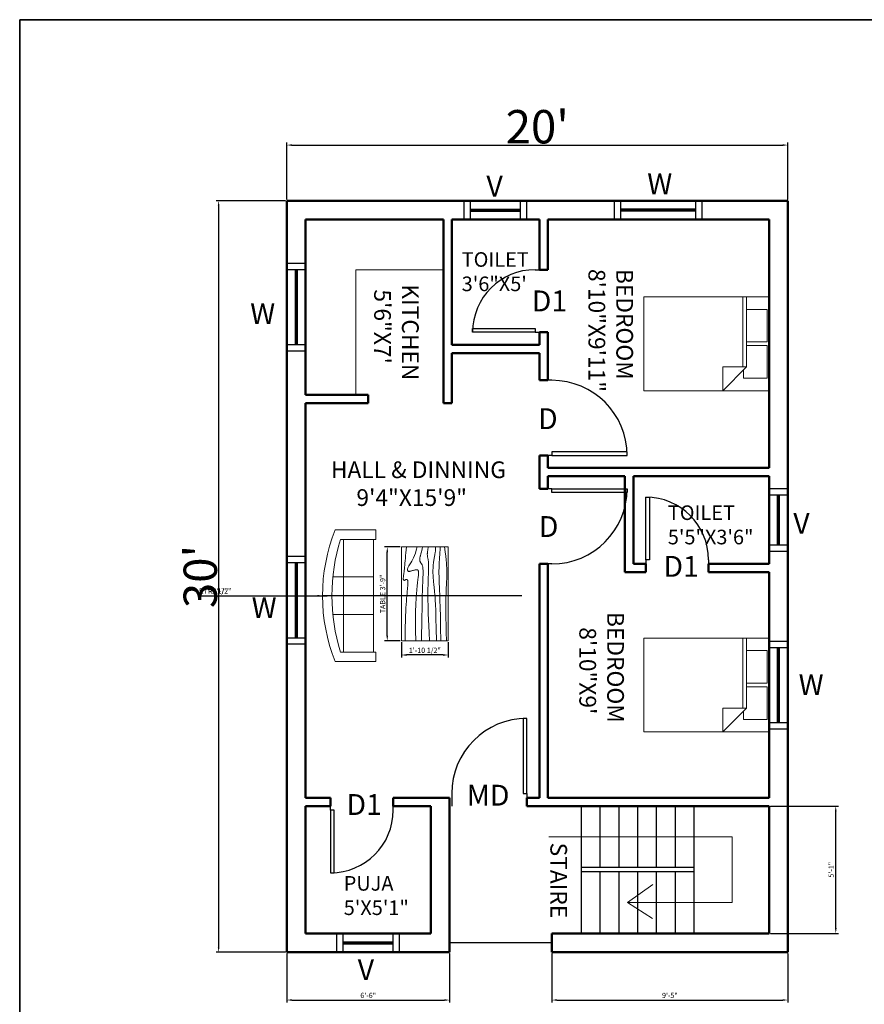
# Model space of a CAD drawing. Units: inches. Extents: x 2150 to 10686, y 1035 to 5077.
# Tile 8 of 12: x 6113 to 6517, y 4605 to 5077. Entities that reach past the tile are written whole.
import ezdxf

# ---------------------------------------------------------------- set-up
doc = ezdxf.new("R2010")
doc.units = ezdxf.units.IN
for name, color, linetype, lineweight in [('A-ANNO-DIMS', 2, 'Continuous', 18), ('A-ANNO-IDEN', 2, 'Continuous', 18), ('A-ANNO-SYMB', 3, 'Continuous', 18), ('A-ANNO-TTLB', 7, 'Continuous', 35), ('A-AREA-IDEN', 7, 'Continuous', 18), ('A-DOOR', 4, 'Continuous', 25), ('A-FLOR-FIXT', 9, 'Continuous', 18), ('A-FLOR-STRS', 4, 'Continuous', 25), ('A-FURN', 8, 'Continuous', 18), ('A-GLAZ', 30, 'Continuous', 25), ('A-WALL', 18, 'Continuous', 50)]:
    doc.layers.add(name, color=color, linetype=linetype, lineweight=lineweight)
doc.styles.get("Standard").update_dxf_attribs({"font": 'arial.ttf'})
doc.dimstyles.new('ISO-25', dxfattribs={"dimtxt": 2.5, "dimasz": 2.5, "dimexe": 1.25, "dimexo": 0.625, "dimtad": 1, "dimdec": 0, "dimlunit": 3, "dimtxsty": 'Standard', "dimcen": 2.5, "dimadec": 0, "dimazin": 0, "dimtfac": 1, "dimtdec": 0, "dimtmove": 0, "dimatfit": 3, "dimfxl": 1, "dimarcsym": 0})

# ---------------------------------------------------------------- blocks, each defined once
blk = doc.blocks.new('*U9')
for p, q in [((0, 0), (0, -6)), ((-36, 0), (-36, -6))]:
    blk.add_line(p, q)
blk.add_lwpolyline([(0, 0), (0, 36), (-1.75, 36), (-1.75, 0)], close=True)
blk.add_arc((0, 0), 36, 90, 180)
blk = doc.blocks.new('*U18')
for p, q in [((0, 0), (0, -6)), ((30, 0), (30, -6))]:
    blk.add_line(p, q)
blk.add_lwpolyline([(0, 0), (0, 30), (1.75, 30), (1.75, 0)], close=True)
blk.add_arc((0, 0), 30, 0, 90)
blk = doc.blocks.new('*U19')
for p, q in [((0, 0), (0, -6)), ((36, 0), (36, -6))]:
    blk.add_line(p, q)
blk.add_lwpolyline([(0, 0), (0, 36), (1.75, 36), (1.75, 0)], close=True)
blk.add_arc((0, 0), 36, 0, 90)
blk = doc.blocks.new('*U20')
for p, q in [((-30, 0), (-30, 6)), ((0, 0), (0, 6))]:
    blk.add_line(p, q)
blk.add_lwpolyline([(0, 0), (0, -30), (-1.75, -30), (-1.75, 0)], close=True)
blk.add_arc((0, 0), 30, 180, 270)
blk = doc.blocks.new('*U21')
for p, q in [((0, 0), (0, 6)), ((30, 0), (30, 6))]:
    blk.add_line(p, q)
blk.add_lwpolyline([(0, 0), (0, -30), (1.75, -30), (1.75, 0)], close=True)
blk.add_arc((0, 0), 30, 270, 0)
blk = doc.blocks.new('Bed - Queen')
for p, q in [((0, -80.00003), (0, 0)), ((0, 0), (59.99999, 0)), ((59.99999, 0), (59.99999, -80.00003)), ((7.99999, -1.2), (28.79998, -1.2)), ((7.99999, -14.4), (7.99999, -1.2)), ((28.79998, -1.2), (28.79998, -14.4)), ((31.19999, -1.2), (51.99999, -1.2)), ((31.19999, -14.4), (31.19999, -1.2)), ((51.99999, -1.2), (51.99999, -16.4)), ((0, -14.4), (44.8, -14.4)), ((44.8, -16.8), (0, -16.8)), ((59.99999, -29.6), (44.8, -14.4)), ((44.8, -14.4), (44.8, -29.6)), ((51.99999, -16.4), (46.79936, -16.4)), ((44.8, -29.6), (59.99999, -29.6)), ((59.99999, -80.00003), (0, -80.00003))]:
    blk.add_line(p, q)
blk = doc.blocks.new('Sofa - Roundback 7 ft.')
for p, q in [((-36.000027, -34), (-36.000027, -11.4696)), ((-12.00002, -32.4421), (-12.00003, -6.5971)), ((11.99997, -32.4421), (11.99998, -6.5971)), ((35.99998, -34), (35.99998, -11.4696)), ((-35.999844, -13.3819), (35.9998, -13.3819)), ((-36.000027, -32.4421), (35.99998, -32.4421))]:
    blk.add_line(p, q)
for points in [[(-36.000027, -34), (-42.000027, -34), (-42.000027, -8)], [(41.99998, -8), (41.99998, -34), (35.99998, -34)]]:
    blk.add_lwpolyline(points)
for centre, radius, start, end in [((0, -114.25), 114.25, 68.43141, 111.5686), ((-0.00001, -127.1968), 121.1968, 72.72033, 107.2797)]:
    blk.add_arc(centre, radius, start, end)
blk = doc.blocks.new('Table - Rectangular Woodgrain 60 x 30 in.')
for p, q in [((0, 0), (0, -30)), ((60, 0), (0, 0)), ((60, -30), (60, 0)), ((0, -30), (60, -30))]:
    blk.add_line(p, q)
for points in [[(0, -2.4), (4.8155, -2.418), (9.0302, -2.4688), (12.709, -2.5477), (15.9167, -2.65), (18.7181, -2.7711), (21.1781, -2.9063), (23.3616, -3.0508), (25.3333, -3.2), (27.1477, -3.3495), (28.8172, -3.4958), (30.3437, -3.636), (31.7291, -3.7667), (32.9756, -3.8849), (34.0849, -3.9875), (35.059, -4.0714), (35.9, -4.1334), (36.6114, -4.1711), (37.2041, -4.1854), (37.6906, -4.1779), (38.0833, -4.15), (38.3948, -4.1034), (38.6375, -4.0396), (38.8239, -3.9602), (38.9666, -3.8667), (39.0764, -3.7608), (39.1573, -3.6448), (39.2116, -3.521), (39.2416, -3.3917), (39.2498, -3.2593), (39.2385, -3.1261), (39.21, -2.9944), (39.1666, -2.8667), (39.111, -2.7447), (39.0468, -2.6281), (38.978, -2.5163), (38.9083, -2.4083), (38.8418, -2.3035), (38.7823, -2.201), (38.7337, -2.1001), (38.7, -2), (38.6844, -1.9003), (38.6875, -1.8021), (38.7094, -1.707), (38.75, -1.6167), (38.8094, -1.5326), (38.8875, -1.4563), (38.9844, -1.3893), (39.1, -1.3333), (39.2351, -1.2896), (39.3937, -1.2583), (39.5804, -1.2396), (39.8, -1.2333), (40.057, -1.2396), (40.3562, -1.2583), (40.7023, -1.2896), (41.1, -1.3333), (41.5547, -1.3895), (42.0755, -1.4573), (42.6721, -1.5361), (43.3542, -1.625), (44.1316, -1.7233), (45.014, -1.8302), (46.0114, -1.9449), (47.1333, -2.0667), (48.3862, -2.1947), (49.7625, -2.3281), (51.2513, -2.4663), (52.8416, -2.6083), (54.5226, -2.7535), (56.2833, -2.9011), (58.1127, -3.0501), (60, -3.2)], [(0, -9.2), (6.5759, -9.0858), (11.9385, -9.0365), (16.2527, -9.0418), (19.6833, -9.0917), (22.3952, -9.1759), (24.5531, -9.2844), (26.322, -9.4069), (27.8666, -9.5333), (29.3241, -9.6553), (30.7203, -9.7719), (32.0532, -9.8837), (33.3208, -9.9917), (34.5213, -10.0965), (35.6526, -10.199), (36.7128, -10.2999), (37.7, -10.4), (38.6129, -10.4996), (39.4531, -10.5969), (40.223, -10.6895), (40.925, -10.775), (41.5613, -10.8512), (42.1344, -10.9156), (42.6465, -10.966), (43.1, -11), (43.4976, -11.0158), (43.8437, -11.0136), (44.143, -10.9942), (44.4, -10.9583), (44.6195, -10.9069), (44.8062, -10.8406), (44.9648, -10.7603), (45.1, -10.6667), (45.2155, -10.5598), (45.3114, -10.4365), (45.3871, -10.2929), (45.4416, -10.125), (45.4743, -9.929), (45.4844, -9.7011), (45.4709, -9.4371), (45.4333, -9.1333), (45.3716, -8.7883), (45.2896, -8.4104), (45.1919, -8.0107), (45.0833, -7.6), (44.9685, -7.1893), (44.8521, -6.7896), (44.7388, -6.4117), (44.6333, -6.0667), (44.54, -5.7628), (44.4614, -5.4979), (44.4001, -5.2675), (44.3583, -5.0667), (44.3384, -4.8909), (44.3427, -4.7354), (44.3736, -4.5956), (44.4333, -4.4667), (44.5236, -4.3453), (44.6427, -4.2333), (44.7884, -4.1339), (44.9583, -4.05), (45.1501, -3.9849), (45.3614, -3.9417), (45.59, -3.9234), (45.8333, -3.9333), (46.0915, -3.9749), (46.3734, -4.0531), (46.6906, -4.1736), (47.0542, -4.3417), (47.4756, -4.5629), (47.9661, -4.8427), (48.5372, -5.1866), (49.2, -5.6), (49.9676, -6.0844), (50.8594, -6.625), (51.8965, -7.2031), (53.1, -7.8), (54.491, -8.3969), (56.0906, -8.975), (57.9199, -9.5156), (60, -10)], [(0, -12.8), (5.1847, -12.9322), (9.6213, -13.0323), (13.3963, -13.1059), (16.5958, -13.1583), (19.3063, -13.1952), (21.614, -13.2219), (23.6054, -13.2439), (25.3666, -13.2667), (26.9728, -13.2947), (28.4531, -13.3281), (29.8256, -13.3663), (31.1083, -13.4083), (32.3191, -13.4535), (33.476, -13.501), (34.597, -13.5501), (35.7, -13.6), (36.7984, -13.6497), (37.8875, -13.6979), (38.9578, -13.743), (40, -13.7833), (41.0047, -13.8174), (41.9625, -13.8438), (42.864, -13.8607), (43.7, -13.8667), (44.4631, -13.8604), (45.1552, -13.8417), (45.7801, -13.8104), (46.3416, -13.7667), (46.8439, -13.7104), (47.2906, -13.6417), (47.6858, -13.5604), (48.0333, -13.4667), (48.3375, -13.3608), (48.6042, -13.2448), (48.8396, -13.121), (49.05, -12.9917), (49.2417, -12.8593), (49.4208, -12.7261), (49.5937, -12.5944), (49.7667, -12.4667), (49.9452, -12.3451), (50.1323, -12.2313), (50.3303, -12.1268), (50.5416, -12.0333), (50.7686, -11.9524), (51.0135, -11.8854), (51.2788, -11.8341), (51.5666, -11.8), (51.8785, -11.7843), (52.2116, -11.7865), (52.562, -11.8059), (52.926, -11.8417), (53.2998, -11.8931), (53.6795, -11.9594), (54.0614, -12.0397), (54.4416, -12.1333), (54.8223, -12.2401), (55.2293, -12.3625), (55.6942, -12.5037), (56.2489, -12.6667), (56.9251, -12.8547), (57.7545, -13.0708), (58.7689, -13.3182), (60, -13.6)], [(0, -18), (5.124, -17.7273), (9.6609, -17.5057), (13.6705, -17.3303), (17.2125, -17.1958), (20.3467, -17.0973), (23.1328, -17.0297), (25.6307, -16.9878), (27.9, -16.9667), (29.9928, -16.9617), (31.9302, -16.9703), (33.7254, -16.9907), (35.3917, -17.0208), (36.9423, -17.0588), (38.3906, -17.1026), (39.7499, -17.1503), (41.0333, -17.2), (42.2519, -17.2496), (43.4073, -17.2969), (44.4986, -17.3395), (45.525, -17.375), (46.4858, -17.4012), (47.3802, -17.4156), (48.2074, -17.416), (48.9667, -17.4), (49.6583, -17.3662), (50.2872, -17.3167), (50.8595, -17.2547), (51.3812, -17.1833), (51.8584, -17.1057), (52.2971, -17.025), (52.7034, -16.9443), (53.0833, -16.8667), (53.443, -16.7951), (53.789, -16.7313), (54.128, -16.6768), (54.4666, -16.6334), (54.8115, -16.6024), (55.1693, -16.5854), (55.5465, -16.5841), (55.95, -16.6), (56.3828, -16.6337), (56.8346, -16.6823), (57.2915, -16.7418), (57.7396, -16.8084), (58.165, -16.878), (58.5539, -16.9469), (58.8924, -17.0111), (59.1666, -17.0667), (59.3679, -17.1107), (59.5078, -17.1438), (59.6032, -17.1675), (59.6708, -17.1833), (59.7275, -17.193), (59.7901, -17.1979), (59.8753, -17.1998), (60, -17.2)], [(0, -22.4), (8.0098, -22.2501), (14.4094, -22.1011), (19.4168, -21.9535), (23.25, -21.8083), (26.1269, -21.6663), (28.2656, -21.5281), (29.884, -21.3947), (31.2, -21.2667), (32.3967, -21.1448), (33.5172, -21.0292), (34.5697, -20.9198), (35.5625, -20.8167), (36.5037, -20.7198), (37.4015, -20.6292), (38.2642, -20.5448), (39.1, -20.4667), (39.9164, -20.3951), (40.7187, -20.3313), (41.5117, -20.2768), (42.3, -20.2333), (43.0883, -20.2024), (43.8812, -20.1854), (44.6836, -20.1841), (45.5, -20.2), (46.3328, -20.234), (47.1747, -20.2844), (48.0163, -20.3488), (48.8479, -20.425), (49.66, -20.5106), (50.4429, -20.6031), (51.1872, -20.7004), (51.8833, -20.8), (52.5246, -20.8999), (53.1166, -20.9995), (53.6681, -21.0983), (54.1875, -21.1958), (54.6834, -21.2919), (55.1646, -21.3859), (55.6394, -21.4777), (56.1167, -21.5667), (56.6028, -21.6515), (57.0961, -21.7266), (57.5929, -21.7852), (58.0896, -21.8208), (58.5823, -21.8268), (59.0674, -21.7964), (59.5412, -21.723), (60, -21.6)], [(0, -25.2), (8.6355, -25.0504), (15.7026, -24.9031), (21.4049, -24.7606), (25.9458, -24.625), (29.529, -24.4988), (32.3578, -24.3844), (34.6359, -24.284), (36.5667, -24.2), (38.3213, -24.1341), (39.9417, -24.0854), (41.437, -24.0523), (42.8167, -24.0333), (44.0901, -24.0268), (45.2667, -24.0313), (46.3557, -24.0451), (47.3667, -24.0667), (48.309, -24.0947), (49.1928, -24.1287), (50.0284, -24.168), (50.826, -24.2125), (51.5959, -24.2617), (52.3483, -24.3151), (53.0935, -24.3725), (53.8417, -24.4334), (54.6009, -24.497), (55.3699, -24.561), (56.1454, -24.6226), (56.9239, -24.6792), (57.7021, -24.7279), (58.4764, -24.7662), (59.2435, -24.7911), (60, -24.8)], [(0, -28.8), (5.6867, -28.6681), (10.45, -28.5698), (14.407, -28.5012), (17.675, -28.4584), (20.3711, -28.4374), (22.6125, -28.4344), (24.5164, -28.4455), (26.2, -28.4667), (27.762, -28.4947), (29.2276, -28.5281), (30.6033, -28.5663), (31.8958, -28.6084), (33.1118, -28.6535), (34.2578, -28.7011), (35.3405, -28.7501), (36.3666, -28.8), (37.3443, -28.8497), (38.288, -28.8974), (39.2137, -28.9412), (40.1375, -28.9792), (41.0753, -29.0093), (42.0432, -29.0297), (43.0572, -29.0384), (44.1333, -29.0333), (45.2936, -29.0114), (46.5843, -28.9641), (48.0579, -28.8816), (49.7666, -28.7542), (51.7629, -28.5721), (54.0989, -28.3255), (56.8272, -28.0048), (60, -27.6)]]:
    blk.add_lwpolyline(points)
blk = doc.blocks.new('*D23')
at = {"layer": 'A-ANNO-DIMS', "color": 0, "lineweight": -2, "transparency": 16777216}
for p, q in [((6240.61, 4990.45), (6240.61, 5017.78)), ((6243.11, 5016.53), (6478.11, 5016.53)), ((6480.61, 4990.45), (6480.61, 5017.78))]:
    blk.add_line(p, q, dxfattribs=at)
at = {"layer": 'A-ANNO-DIMS', "color": 0, "transparency": 16777216}
for points in [[(6243.11, 5016.94), (6243.11, 5016.11), (6240.61, 5016.53)], [(6478.11, 5016.94), (6478.11, 5016.11), (6480.61, 5016.53)]]:
    blk.add_solid(points, dxfattribs=at)
at = {"layer": 'Defpoints', "color": 0, "transparency": 16777216}
for p in [(6480.61, 5016.53), (6240.61, 4989.82), (6480.61, 4989.82)]:
    blk.add_point(p, dxfattribs=at)
at = {"layer": 'A-ANNO-DIMS', "color": 0, "transparency": 16777216, "insert": (6360.61, 5025.32), "char_height": 2.5, "attachment_point": 5}
blk.add_mtext("{\\H6.4x;20'}", dxfattribs=at)
blk = doc.blocks.new('*D24')
at = {"layer": 'A-ANNO-DIMS', "color": 0, "lineweight": -2, "transparency": 16777216}
for p, q in [((6239.98, 4989.82), (6206.73, 4989.82)), ((6207.98, 4987.32), (6207.98, 4632.32)), ((6239.98, 4629.82), (6206.73, 4629.82))]:
    blk.add_line(p, q, dxfattribs=at)
at = {"layer": 'A-ANNO-DIMS', "color": 0, "transparency": 16777216}
for points in [[(6207.56, 4987.32), (6208.39, 4987.32), (6207.98, 4989.82)], [(6207.56, 4632.32), (6208.39, 4632.32), (6207.98, 4629.82)]]:
    blk.add_solid(points, dxfattribs=at)
at = {"layer": 'Defpoints', "color": 0, "transparency": 16777216}
for p in [(6240.61, 4989.82), (6207.98, 4629.82), (6240.61, 4629.82)]:
    blk.add_point(p, dxfattribs=at)
at = {"layer": 'A-ANNO-DIMS', "color": 0, "transparency": 16777216, "insert": (6199.18, 4809.82), "char_height": 2.5, "attachment_point": 5, "rotation": 90}
blk.add_mtext("{\\H6.4x;30'}", dxfattribs=at)
blk = doc.blocks.new('WINDOW-36IN')
for p, q in [((9, 42), (0, 42)), ((9, 39), (0, 39)), ((4, 39), (4, 3)), ((4.5, 39), (4.5, 3)), ((5, 39), (5, 3)), ((9, 3), (0, 3)), ((9, 0), (0, 0))]:
    blk.add_line(p, q)
blk = doc.blocks.new('VENT-24IN')
for p, q in [((0, 30), (9, 30)), ((0, 27), (9, 27)), ((4, 27), (4, 3)), ((4.5, 27), (4.5, 3)), ((5, 27), (5, 3)), ((0, 3), (9, 3)), ((0, 0), (9, 0))]:
    blk.add_line(p, q)
blk = doc.blocks.new('*D62')
at = {"layer": 'A-ANNO-DIMS', "color": 0, "lineweight": -2, "transparency": 16777216}
for p, q in [((6294.87, 4823.95), (6287.49, 4823.95)), ((6288.74, 4781.45), (6288.74, 4821.45)), ((6294.87, 4778.95), (6287.49, 4778.95))]:
    blk.add_line(p, q, dxfattribs=at)
at = {"layer": 'A-ANNO-DIMS', "color": 0, "transparency": 16777216}
for points in [[(6288.33, 4821.45), (6289.16, 4821.45), (6288.74, 4823.95)], [(6288.33, 4781.45), (6289.16, 4781.45), (6288.74, 4778.95)]]:
    blk.add_solid(points, dxfattribs=at)
at = {"layer": 'Defpoints', "color": 0, "transparency": 16777216}
for p in [(6288.74, 4823.95), (6295.49, 4823.95), (6295.49, 4778.95)]:
    blk.add_point(p, dxfattribs=at)
at = {"layer": 'A-ANNO-DIMS', "color": 0, "transparency": 16777216, "insert": (6286.84, 4801.45), "char_height": 2.5, "attachment_point": 5, "rotation": 90}
blk.add_mtext('TABLE 3\'-9"', dxfattribs=at)
blk = doc.blocks.new('*D63')
at = {"layer": 'A-ANNO-DIMS', "color": 0, "lineweight": -2, "transparency": 16777216}
for p, q in [((6295.49, 4778.32), (6295.49, 4770.95)), ((6317.99, 4778.32), (6317.99, 4770.95)), ((6315.49, 4772.2), (6297.99, 4772.2))]:
    blk.add_line(p, q, dxfattribs=at)
at = {"layer": 'A-ANNO-DIMS', "color": 0, "transparency": 16777216}
for points in [[(6297.99, 4772.61), (6297.99, 4771.78), (6295.49, 4772.2)], [(6315.49, 4772.61), (6315.49, 4771.78), (6317.99, 4772.2)]]:
    blk.add_solid(points, dxfattribs=at)
at = {"layer": 'Defpoints', "color": 0, "transparency": 16777216}
for p in [(6295.49, 4778.95), (6317.99, 4778.95), (6295.49, 4772.2)]:
    blk.add_point(p, dxfattribs=at)
at = {"layer": 'A-ANNO-DIMS', "color": 0, "transparency": 16777216, "insert": (6306.74, 4774.11), "char_height": 2.5, "attachment_point": 5}
blk.add_mtext('1\'-10 1/2"', dxfattribs=at)
blk = doc.blocks.new('*D144')
at = {"layer": 'A-ANNO-DIMS', "color": 0, "lineweight": -2, "transparency": 16777216}
for p, q in [((6240.61, 4629.2), (6240.61, 4605.62)), ((6318.61, 4629.2), (6318.61, 4605.62)), ((6243.11, 4606.87), (6316.11, 4606.87))]:
    blk.add_line(p, q, dxfattribs=at)
at = {"layer": 'A-ANNO-DIMS', "color": 0, "transparency": 16777216}
for points in [[(6243.11, 4607.29), (6243.11, 4606.46), (6240.61, 4606.87)], [(6316.11, 4607.29), (6316.11, 4606.46), (6318.61, 4606.87)]]:
    blk.add_solid(points, dxfattribs=at)
at = {"layer": 'Defpoints', "color": 0, "transparency": 16777216}
for p in [(6240.61, 4629.82), (6318.61, 4629.82), (6318.61, 4606.87)]:
    blk.add_point(p, dxfattribs=at)
at = {"layer": 'A-ANNO-DIMS', "color": 0, "transparency": 16777216, "insert": (6279.61, 4608.77), "char_height": 2.5, "attachment_point": 5}
blk.add_mtext('6\'-6"', dxfattribs=at)
blk = doc.blocks.new('*D145')
at = {"layer": 'A-ANNO-DIMS', "color": 0, "lineweight": -2, "transparency": 16777216}
for p, q in [((6367.61, 4629.2), (6367.61, 4605.62)), ((6480.61, 4629.2), (6480.61, 4605.62)), ((6370.11, 4606.87), (6478.11, 4606.87))]:
    blk.add_line(p, q, dxfattribs=at)
at = {"layer": 'A-ANNO-DIMS', "color": 0, "transparency": 16777216}
for points in [[(6370.11, 4607.29), (6370.11, 4606.46), (6367.61, 4606.87)], [(6478.11, 4607.29), (6478.11, 4606.46), (6480.61, 4606.87)]]:
    blk.add_solid(points, dxfattribs=at)
at = {"layer": 'Defpoints', "color": 0, "transparency": 16777216}
for p in [(6367.61, 4629.82), (6480.61, 4629.82), (6480.61, 4606.87)]:
    blk.add_point(p, dxfattribs=at)
at = {"layer": 'A-ANNO-DIMS', "color": 0, "transparency": 16777216, "insert": (6424.11, 4608.77), "char_height": 2.5, "attachment_point": 5}
blk.add_mtext('9\'-5"', dxfattribs=at)
blk = doc.blocks.new('*D146')
at = {"layer": 'A-ANNO-DIMS', "color": 0, "lineweight": -2, "transparency": 16777216}
for p, q in [((6472.23, 4699.82), (6504.81, 4699.82)), ((6503.56, 4641.32), (6503.56, 4697.32)), ((6472.23, 4638.82), (6504.81, 4638.82))]:
    blk.add_line(p, q, dxfattribs=at)
at = {"layer": 'A-ANNO-DIMS', "color": 0, "transparency": 16777216}
for points in [[(6503.14, 4697.32), (6503.97, 4697.32), (6503.56, 4699.82)], [(6503.14, 4641.32), (6503.97, 4641.32), (6503.56, 4638.82)]]:
    blk.add_solid(points, dxfattribs=at)
at = {"layer": 'Defpoints', "color": 0, "transparency": 16777216}
for p in [(6471.61, 4699.82), (6503.56, 4699.82), (6471.61, 4638.82)]:
    blk.add_point(p, dxfattribs=at)
at = {"layer": 'A-ANNO-DIMS', "color": 0, "transparency": 16777216, "insert": (6501.66, 4669.32), "char_height": 2.5, "attachment_point": 5, "rotation": 90}
blk.add_mtext('5\'-1"', dxfattribs=at)
blk = doc.blocks.new('*D155')
at = {"layer": 'A-ANNO-DIMS', "color": 0, "lineweight": -2, "transparency": 16777216}
for p, q in [((6202.56, 4800.61), (6259.74, 4800.61)), ((6353.14, 4800.61), (6262.24, 4800.61))]:
    blk.add_line(p, q, dxfattribs=at)
at = {"layer": 'A-ANNO-DIMS', "color": 0, "transparency": 16777216}
blk.add_solid([(6259.74, 4801.02), (6259.74, 4800.19), (6262.24, 4800.61)], dxfattribs=at)
at = {"layer": 'Defpoints', "color": 0, "transparency": 16777216}
for p in [(6262.24, 4800.61), (6353.14, 4800.61)]:
    blk.add_point(p, dxfattribs=at)
at = {"layer": 'A-ANNO-DIMS', "color": 0, "transparency": 16777216, "insert": (6207.7, 4802.48), "char_height": 2.5, "attachment_point": 5, "rotation": 0.0001}
blk.add_mtext('R7\'-7"', dxfattribs=at)
blk = doc.blocks.new('*D156')
at = {"layer": 'A-ANNO-DIMS', "color": 0, "lineweight": -2, "transparency": 16777216}
for p, q in [((6198.27, 4800.61), (6255.24, 4800.61)), ((6343.43, 4800.61), (6257.74, 4800.61))]:
    blk.add_line(p, q, dxfattribs=at)
at = {"layer": 'A-ANNO-DIMS', "color": 0, "transparency": 16777216}
blk.add_solid([(6255.24, 4801.02), (6255.24, 4800.19), (6257.74, 4800.61)], dxfattribs=at)
at = {"layer": 'Defpoints', "color": 0, "transparency": 16777216}
for p in [(6257.74, 4800.61), (6343.43, 4800.61)]:
    blk.add_point(p, dxfattribs=at)
at = {"layer": 'A-ANNO-DIMS', "color": 0, "transparency": 16777216, "insert": (6206.33, 4802.53), "char_height": 2.5, "attachment_point": 5, "rotation": 0.0001}
blk.add_mtext('R7\'-1 1/2"', dxfattribs=at)

msp = doc.modelspace()

# ---------------------------------------------------------------- linework, layer by layer
at = {"layer": 'A-ANNO-SYMB'}
for p, q in [((6366.07, 4685.07), (6453.96, 4685.07)), ((6453.96, 4685.07), (6453.96, 4653.57)), ((6403.79, 4653.57), (6415.87, 4662.29)), ((6453.96, 4653.57), (6403.79, 4653.57)), ((6403.79, 4653.57), (6415.82, 4645.99))]:
    msp.add_line(p, q, dxfattribs=at)
at = {"layer": 'A-ANNO-TTLB'}
msp.add_lwpolyline([(6112.69, 5076.61), (7001.25, 5076.61), (7001.25, 4201.35), (6112.69, 4201.35)], close=True, dxfattribs=at)
at = {"layer": 'A-DOOR'}
msp.add_line((6367.61, 4634.32), (6318.61, 4634.32), dxfattribs=at)
at = {"layer": 'A-FLOR-FIXT'}
for p, q in [((6273.61, 4896.82), (6273.61, 4956.82)), ((6273.61, 4956.82), (6315.61, 4956.82))]:
    msp.add_line(p, q, dxfattribs=at)
at = {"layer": 'A-FLOR-STRS'}
for p, q in [((6381.61, 4699.82), (6381.61, 4670.32)), ((6390.61, 4699.82), (6390.61, 4670.32)), ((6399.61, 4699.82), (6399.61, 4670.32)), ((6408.61, 4699.82), (6408.61, 4670.32)), ((6417.61, 4699.82), (6417.61, 4670.32)), ((6426.61, 4699.82), (6426.61, 4670.32)), ((6435.61, 4699.82), (6435.61, 4638.82)), ((6435.61, 4670.32), (6381.61, 4670.32)), ((6381.61, 4670.32), (6381.61, 4638.82)), ((6435.61, 4668.32), (6381.61, 4668.32)), ((6390.61, 4668.32), (6390.61, 4638.82)), ((6399.61, 4668.32), (6399.61, 4638.82)), ((6408.61, 4668.32), (6408.61, 4638.82)), ((6417.61, 4668.32), (6417.61, 4638.82)), ((6426.61, 4668.32), (6426.61, 4638.82))]:
    msp.add_line(p, q, dxfattribs=at)
at = {"layer": 'A-WALL'}
for p, q in [((6240.61, 4989.82), (6480.61, 4989.82)), ((6240.61, 4629.82), (6240.61, 4989.82)), ((6480.61, 4989.82), (6480.61, 4629.82)), ((6249.61, 4980.82), (6315.61, 4980.82)), ((6249.61, 4896.82), (6249.61, 4980.82)), ((6315.61, 4892.82), (6315.61, 4980.82)), ((6319.61, 4920.82), (6319.61, 4980.82)), ((6319.61, 4980.82), (6361.61, 4980.82)), ((6361.61, 4956.82), (6361.61, 4980.82)), ((6365.61, 4956.82), (6365.61, 4980.82)), ((6365.61, 4980.82), (6471.61, 4980.82)), ((6471.61, 4980.82), (6471.61, 4861.82)), ((6361.61, 4956.82), (6365.61, 4956.82)), ((6361.61, 4926.82), (6365.61, 4926.82)), ((6361.61, 4920.82), (6361.61, 4926.82)), ((6365.61, 4903.82), (6365.61, 4926.82)), ((6319.61, 4920.82), (6361.61, 4920.82)), ((6319.61, 4916.82), (6361.61, 4916.82)), ((6319.61, 4892.82), (6319.61, 4916.82)), ((6361.61, 4903.82), (6361.61, 4916.82)), ((6361.61, 4903.82), (6365.61, 4903.82)), ((6249.61, 4896.82), (6279.61, 4896.82)), ((6249.61, 4892.82), (6279.61, 4892.82)), ((6249.61, 4703.82), (6249.61, 4892.82)), ((6279.61, 4892.82), (6279.61, 4896.82)), ((6315.61, 4892.82), (6319.61, 4892.82)), ((6361.61, 4851.82), (6361.61, 4867.82)), ((6361.61, 4867.82), (6365.61, 4867.82)), ((6365.61, 4861.82), (6365.61, 4867.82)), ((6365.61, 4861.82), (6471.61, 4861.82)), ((6365.61, 4857.82), (6402.61, 4857.82)), ((6365.61, 4851.82), (6365.61, 4857.82)), ((6402.61, 4857.82), (6402.61, 4811.82)), ((6406.61, 4857.82), (6406.61, 4815.82)), ((6406.61, 4857.82), (6471.61, 4857.82)), ((6471.61, 4857.82), (6471.61, 4815.82)), ((6361.61, 4851.82), (6365.61, 4851.82)), ((6361.61, 4703.82), (6361.61, 4815.82)), ((6361.61, 4815.82), (6365.61, 4815.82)), ((6365.61, 4703.82), (6365.61, 4815.82)), ((6406.61, 4815.82), (6412.61, 4815.82)), ((6412.61, 4815.82), (6412.61, 4811.82)), ((6442.61, 4815.82), (6442.61, 4811.82)), ((6442.61, 4815.82), (6471.61, 4815.82)), ((6402.61, 4811.82), (6412.61, 4811.82)), ((6442.61, 4811.82), (6471.61, 4811.82)), ((6471.61, 4811.82), (6471.61, 4703.82)), ((6249.61, 4703.82), (6261.61, 4703.82)), ((6261.61, 4699.82), (6261.61, 4703.82)), ((6291.61, 4699.82), (6291.61, 4703.82)), ((6291.61, 4703.82), (6318.61, 4703.82)), ((6318.61, 4629.82), (6318.61, 4703.82)), ((6355.61, 4699.82), (6355.61, 4703.82)), ((6355.61, 4703.82), (6361.61, 4703.82)), ((6365.61, 4703.82), (6471.61, 4703.82)), ((6249.61, 4638.82), (6249.61, 4699.82)), ((6309.61, 4638.82), (6309.61, 4699.82)), ((6471.61, 4699.82), (6471.61, 4638.82)), ((6309.61, 4638.82), (6249.61, 4638.82)), ((6471.61, 4638.82), (6367.61, 4638.82)), ((6367.61, 4638.82), (6367.61, 4629.82)), ((6318.61, 4629.82), (6240.61, 4629.82)), ((6480.61, 4629.82), (6367.61, 4629.82))]:
    msp.add_line(p, q, dxfattribs=at)
for points in [[(6249.61, 4699.82), (6261.61, 4699.82)], [(6291.61, 4699.82), (6309.61, 4699.82)], [(6355.61, 4699.82), (6471.61, 4699.82)]]:
    msp.add_lwpolyline(points, dxfattribs=at)

# ---------------------------------------------------------------- block references
at = {"layer": 'A-DOOR', "rotation": 270}
for name, p in [('*U20', (6359.61, 4926.82)), ('*U9', (6367.61, 4867.82)), ('*U19', (6367.61, 4851.82))]:
    msp.add_blockref(name, p, dxfattribs=at)
at = {"layer": 'A-DOOR'}
for name, p in [('*U18', (6412.61, 4817.82)), ('*U9', (6355.61, 4705.82)), ('*U21', (6261.61, 4697.82))]:
    msp.add_blockref(name, p, dxfattribs=at)
at = {"layer": 'A-FURN', "xscale": 0.75, "yscale": 0.75, "zscale": 0.75}
for name, p, rotation in [('Bed - Queen', (6471.61, 4943.82), 270), ('Sofa - Roundback 7 ft.', (6257.74, 4800.61), 90), ('Table - Rectangular Woodgrain 60 x 30 in.', (6295.49, 4778.95), 90), ('Bed - Queen', (6471.61, 4780.32), 270)]:
    msp.add_blockref(name, p, dxfattribs=dict(at, rotation=rotation))
at = {"layer": 'A-GLAZ'}
for name, p, rotation in [('VENT-24IN', (6355.61, 4980.82), 90.000000000002), ('WINDOW-36IN', (6397.61, 4989.82), 269.999999999997), ('VENT-24IN', (6480.61, 4851.82), 180), ('WINDOW-36IN', (6480.61, 4778.82), 180), ('VENT-24IN', (6294.61, 4629.82), 90.00000000000296)]:
    msp.add_blockref(name, p, dxfattribs=dict(at, rotation=rotation))
for p in [(6240.61, 4917.82), (6240.61, 4777.32)]:
    msp.add_blockref('WINDOW-36IN', p, dxfattribs=at)

# ---------------------------------------------------------------- texts
at = {"layer": 'A-ANNO-IDEN', "char_height": 10, "attachment_point": 1}
for s, insert in [('V', (6336.23, 5001.89)), ('W', (6413.27, 5002.96)), ('D1', (6357.94, 4946.86)), ('W', (6223.09, 4940.77)), ('D', (6360.97, 4890.41)), ('D', (6361.33, 4838.74)), ('V', (6483.21, 4840.3)), ('D1', (6421.02, 4819.66)), ('W', (6223.79, 4799.9)), ('W', (6485.77, 4763)), ('MD', (6326.82, 4710.02)), ('D1', (6269.2, 4705.55)), ('V', (6274.58, 4626.41))]:
    msp.add_mtext_dynamic_manual_height_columns(s, width=211.6609, gutter_width=12.5, heights=[0], dxfattribs=dict(at, insert=insert))
at = {"layer": 'A-AREA-IDEN', "attachment_point": 1}
for s, width, insert, char_height in [('TOILET\\P3\'6"X5\'', 392.7267, (6324.39, 4965.21), 7), ('HALL & DINNING\\P     9\'4"X15\'9"', 323.157, (6261.74, 4864.96), 8), ('TOILET\\P5\'5"X3\'6"', 127.1364, (6423.12, 4843.89), 7), ('PUJA\\P5\'X5\'1"', 239.2367, (6267.89, 4666.28), 7)]:
    msp.add_mtext_dynamic_manual_height_columns(s, width=width, gutter_width=12.5, heights=[0], dxfattribs=dict(at, insert=insert, char_height=char_height))
at = {"layer": 'A-AREA-IDEN', "char_height": 8, "attachment_point": 1, "rotation": 270}
for s, width, insert in [('BEDROOM\\P8\'10"X9\'11"', 205.3752, (6406.46, 4957.19)), ('KITCHEN\\P 5\'6"X7\'', 257.167, (6303.8, 4949.82)), ('BEDROOM\\P   8\'10"X9\'', 205.3752, (6402.09, 4792.82)), ('STAIRE', 169.3447, (6374.87, 4682.3))]:
    msp.add_mtext_dynamic_manual_height_columns(s, width=width, gutter_width=12.5, heights=[0], dxfattribs=dict(at, insert=insert))

# ---------------------------------------------------------------- dimensions: what is measured, and where the dimension line sits
at = {"layer": 'A-ANNO-DIMS'}
dim = msp.add_linear_dim(base=(6480.61, 5016.53), p1=(6240.61, 4989.82), p2=(6480.61, 4989.82), text='{\\H6.4x;<>}', dimstyle='ISO-25', override={"dimclrd": 0, "dimclre": 0, "dimclrt": 0}, dxfattribs=at)
dim.commit()
dim.dimension.update_dxf_attribs({"geometry": '*D23', "text_midpoint": (6360.61, 5025.32)})
for base, p1, p2, text, override, picture, middle in [((6207.98, 4629.82), (6240.61, 4989.82), (6240.61, 4629.82), '{\\H6.4x;<>}', {"dimclrd": 0, "dimclre": 0, "dimclrt": 0}, '*D24', (6199.18, 4809.82)), ((6288.74, 4823.95), (6295.49, 4778.95), (6295.49, 4823.95), 'TABLE <>', {"dimdec": 1, "dimlfac": 1, "dimrnd": 0, "dimzin": 1, "dimdsep": 46, "dimlunit": 4, "dimfrac": 2}, '*D62', (6286.84, 4801.45))]:
    dim = msp.add_linear_dim(base=base, p1=p1, p2=p2, angle=90, text=text, dimstyle='ISO-25', override=override, dxfattribs=at)
    dim.commit()
    dim.dimension.update_dxf_attribs({"geometry": picture, "text_midpoint": middle})
for center, mpoint, picture, middle in [((6343.43, 4800.61), (6257.74, 4800.61), '*D156', (6206.33, 4800.61)), ((6353.14, 4800.61), (6262.24, 4800.61), '*D155', (6207.7, 4800.61))]:
    dim = msp.add_radius_dim(center=center, mpoint=mpoint, dimstyle='ISO-25', override={"dimdec": 1, "dimlfac": 1, "dimrnd": 0, "dimzin": 1, "dimdsep": 46, "dimlunit": 4, "dimfrac": 2}, dxfattribs=at)
    dim.commit()
    dim.dimension.update_dxf_attribs({"geometry": picture, "text_midpoint": middle, "dimtype": 164})
for base, p1, p2, angle, picture, middle in [((6295.49, 4772.2), (6317.99, 4778.95), (6295.49, 4778.95), 180, '*D63', (6306.74, 4774.11)), ((6503.56, 4699.82), (6471.61, 4638.82), (6471.61, 4699.82), 90, '*D146', (6501.66, 4669.32))]:
    dim = msp.add_linear_dim(base=base, p1=p1, p2=p2, angle=angle, dimstyle='ISO-25', override={"dimdec": 1, "dimlfac": 1, "dimrnd": 0, "dimzin": 1, "dimdsep": 46, "dimlunit": 4, "dimfrac": 2}, dxfattribs=at)
    dim.commit()
    dim.dimension.update_dxf_attribs({"geometry": picture, "text_midpoint": middle})
for base, p1, p2, picture, middle in [((6318.61, 4606.87), (6240.61, 4629.82), (6318.61, 4629.82), '*D144', (6279.61, 4608.77)), ((6480.61, 4606.87), (6367.61, 4629.82), (6480.61, 4629.82), '*D145', (6424.11, 4608.77))]:
    dim = msp.add_linear_dim(base=base, p1=p1, p2=p2, dimstyle='ISO-25', override={"dimdec": 1, "dimlfac": 1, "dimrnd": 0, "dimzin": 1, "dimdsep": 46, "dimlunit": 4, "dimfrac": 2}, dxfattribs=at)
    dim.commit()
    dim.dimension.update_dxf_attribs({"geometry": picture, "text_midpoint": middle})

doc.saveas('drawing.dxf')
